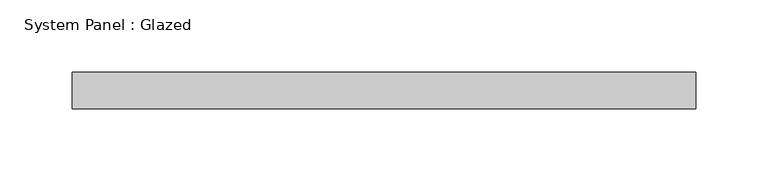
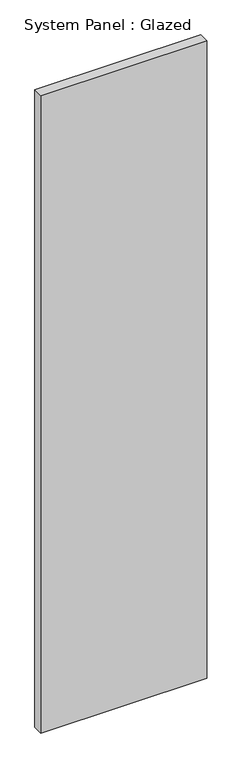
"""IFC4 building model written with IfcOpenShell, lengths in millimetres: plate geometry, System Panel : Glazed."""

from ifc_helpers import new_model, si_unit, origin, origin_with_axes, place, context, project, spatial, polyline, outline, extrude, source, transform, mapped, element, save


def system_panel_glazed_d31e9b5d(model_context):
    return source(origin(), model_context, "Body", "SweptSolid", [
        extrude(outline(polyline([(215.9, 19.05), (-215.9, 19.05), (-215.9, 44.45), (215.9, 44.45), (215.9, 19.05)])), origin_with_axes(), (0.0, 0.0, 1.0), 1752.6),
    ])


if __name__ == "__main__":
    model = new_model("IFC4")
    model_context = context("Model", 3, world=origin())
    ifc_project = project(units=[si_unit("LENGTHUNIT", "METRE", prefix="MILLI")], contexts=[model_context])
    site = spatial("IfcSite", under=ifc_project)
    building = spatial("IfcBuilding", under=site)
    placement = place(None, origin())
    system_panel_glazed_shape = system_panel_glazed_d31e9b5d(model_context)
    element("IfcPlate", 1, ObjectType="System Panel : Glazed", at=placement, inside=building, context=model_context, shape_type="MappedRepresentation", body=[
        mapped(system_panel_glazed_shape, transform((0.0, 0.0, 0.0), x_axis=(1.0, 0.0, 0.0), y_axis=(0.0, 1.0, 0.0), z_axis=(0.0, 0.0, 1.0))),
    ])
    save(model, "model.ifc")

# Revit data of these elements
# Type "System Panel : Glazed"
#   Construction Type Id = "GSP4R"
#   Analytic Construction = "1/8 in Pilkington single glazing"
#   Visual Light Transmittance = 0.9
#   Solar Heat Gain Coefficient = 0.86
#   Heat Transfer Coefficient (U) = 1.18115 BTU/(h·ft²·°F)
#   Define Thermal Properties by = 1
# Element 1 (IfcPlate, "System Panel : Glazed")
#   Materials on its faces: "Glass"
# Materials
#   "Glass": class "Glass", colour RGB 0 128 192, transparency 0.75, Description = "Soda Lime Glass", Cost = 0
